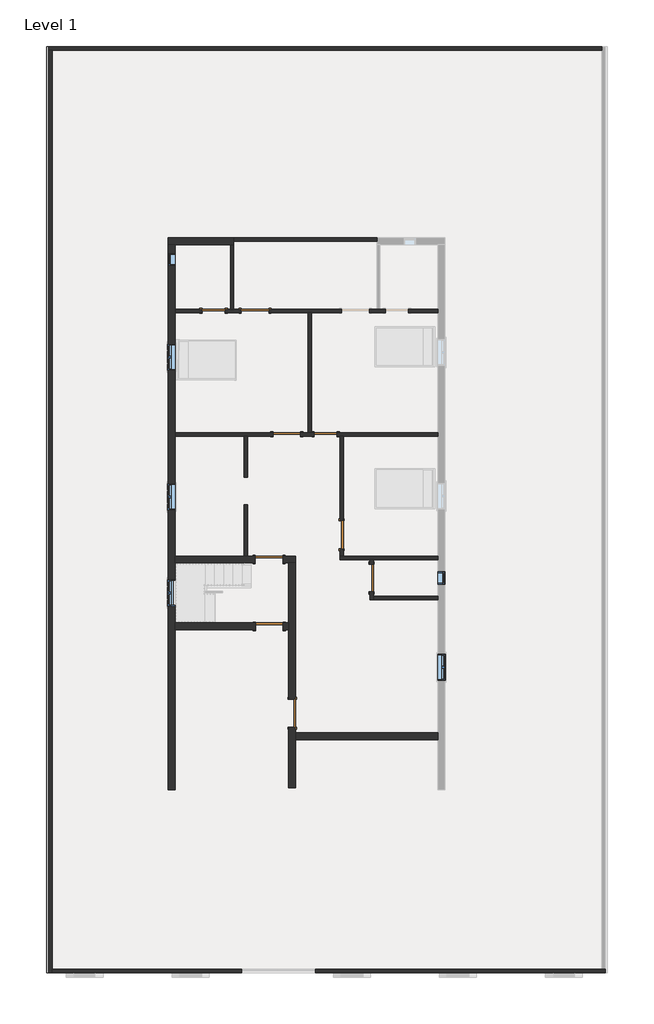
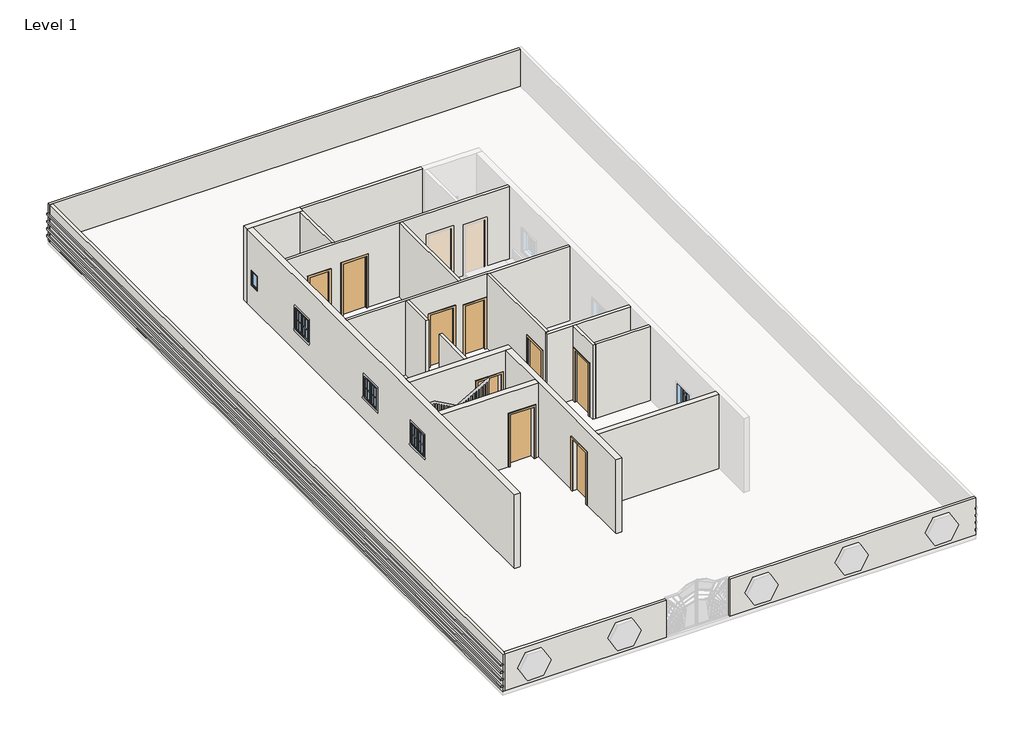
# One storey, part 1 of 3: 21 walls, 9 doors, 6 windows, 4 proxies.
"""IFC4 building model written with IfcOpenShell, lengths in millimetres."""

from ifc_helpers import new_model, si_unit, frame, origin, origin_with_axes, place, context, project, spatial, polyline, outline, extrude, faceted_brep, transform, mapped, element, save
from components import door_d8f5dbb5, door_f2b275c1, door_e5f9f3c4, door_0ca8825f, door_305aa2a5, window_aa618e30, window_339605e1

model = new_model("IFC4")

# Units and contexts
model_context = context("Model", 3, world=origin())
ifc_project = project(units=[si_unit("LENGTHUNIT", "METRE", prefix="MILLI")], contexts=[model_context])

# Site, building, storey
site = spatial("IfcSite", under=ifc_project)
building = spatial("IfcBuilding", under=site)
storey = spatial("IfcBuildingStorey", under=building, Name="Level 1", Elevation=0.0)

# Proxies
placement = place(None, origin())
element("IfcBuildingElementProxy", 1, Name="Reveal", ObjectType="Reveal", at=placement, inside=storey, context=model_context, shape_type="SweptSolid", body=[
    extrude(outline(polyline([(-9754.4734646, -13853.8284905), (-9846.5484646, -13853.8284905), (-9846.5484646, 16740.4715095), (-9754.4734646, 16740.4715095), (-9754.4734646, -13853.8284905)])), frame((0.0, 0.0, 1066.8), z_axis=(0.0, 0.0, 1.0), x_axis=(1.0, 0.0, 0.0)), (0.0, 0.0, 1.0), 67.7333333),
])
element("IfcBuildingElementProxy", 2, Name="Reveal", ObjectType="Reveal", at=placement, inside=storey, context=model_context, shape_type="SweptSolid", body=[
    extrude(outline(polyline([(-9754.4734646, -13853.8284905), (-9846.5484646, -13853.8284905), (-9846.5484646, 16740.4715095), (-9754.4734646, 16740.4715095), (-9754.4734646, -13853.8284905)])), frame((0.0, 0.0, 765.4296979), z_axis=(0.0, 0.0, 1.0), x_axis=(1.0, 0.0, 0.0)), (0.0, 0.0, 1.0), 67.7333333),
])
element("IfcBuildingElementProxy", 3, Name="Reveal", ObjectType="Reveal", at=placement, inside=storey, context=model_context, shape_type="SweptSolid", body=[
    extrude(outline(polyline([(-9754.4734646, -13853.8284905), (-9846.5484646, -13853.8284905), (-9846.5484646, 16740.4715095), (-9754.4734646, 16740.4715095), (-9754.4734646, -13853.8284905)])), frame((0.0, 0.0, 464.0593958), z_axis=(0.0, 0.0, 1.0), x_axis=(1.0, 0.0, 0.0)), (0.0, 0.0, 1.0), 67.7333333),
])
element("IfcBuildingElementProxy", 4, Name="Reveal", ObjectType="Reveal", at=placement, inside=storey, context=model_context, shape_type="SweptSolid", body=[
    extrude(outline(polyline([(-9754.4734646, -13853.8284905), (-9846.5484646, -13853.8284905), (-9846.5484646, 16740.4715095), (-9754.4734646, 16740.4715095), (-9754.4734646, -13853.8284905)])), frame((0.0, 0.0, 174.9956289), z_axis=(0.0, 0.0, 1.0), x_axis=(1.0, 0.0, 0.0)), (0.0, 0.0, 1.0), 67.7333333),
])

# Doors
door_shape = door_d8f5dbb5(model_context)
element("IfcDoor", 5, ObjectType="Single-Flush : 30\" x 80\"", at=placement, inside=storey, context=model_context, shape_type="MappedRepresentation", body=[
    mapped(door_shape, transform((-4322.2915084, 8007.7072267, 0.0), x_axis=(1.0, 0.0, 0.0), y_axis=(0.0, 1.0, 0.0), z_axis=(0.0, 0.0, 1.0))),
])
door_2_shape = door_f2b275c1(model_context)
element("IfcDoor", 6, ObjectType="Single-Flush : 30\" x 80\"", at=placement, inside=storey, context=model_context, shape_type="MappedRepresentation", body=[
    mapped(door_2_shape, transform((-621.124692, 3931.0072267, 0.0), x_axis=(-1.0, 0.0, 0.0), y_axis=(0.0, -1.0, 0.0), z_axis=(0.0, 0.0, 1.0))),
])
door_3_shape = door_e5f9f3c4(model_context)
element("IfcDoor", 7, ObjectType="Single-Flush : 36\" x 84\"", at=placement, inside=storey, context=model_context, shape_type="MappedRepresentation", body=[
    mapped(door_3_shape, transform((-1909.2915084, 3931.0072267, 0.0), x_axis=(1.0, 0.0, 0.0), y_axis=(0.0, 1.0, 0.0), z_axis=(0.0, 0.0, 1.0))),
])
element("IfcDoor", 8, ObjectType="Single-Flush : 36\" x 84\"", at=placement, inside=storey, context=model_context, shape_type="MappedRepresentation", body=[
    mapped(door_3_shape, transform((-94.9578757, 616.3072267, 0.0), x_axis=(0.0, -1.0, 0.0), y_axis=(1.0, 0.0, 0.0), z_axis=(0.0, 0.0, 1.0))),
])
door_4_shape = door_0ca8825f(model_context)
element("IfcDoor", 9, ObjectType="Single-Flush : 36\" x 84\"", at=placement, inside=storey, context=model_context, shape_type="MappedRepresentation", body=[
    mapped(door_4_shape, transform((-2490.3165084, -202.8427733, 0.0), x_axis=(1.0, 0.0, 0.0), y_axis=(0.0, 1.0, 0.0), z_axis=(0.0, 0.0, 1.0))),
])
element("IfcDoor", 10, ObjectType="Single-Flush : 36\" x 84\"", at=placement, inside=storey, context=model_context, shape_type="MappedRepresentation", body=[
    mapped(door_4_shape, transform((-2487.1415084, -2412.6427733, 0.0), x_axis=(1.0, 0.0, 0.0), y_axis=(0.0, 1.0, 0.0), z_axis=(0.0, 0.0, 1.0))),
])
element("IfcDoor", 11, ObjectType="Single-Flush : 36\" x 84\"", at=placement, inside=storey, context=model_context, shape_type="MappedRepresentation", body=[
    mapped(door_4_shape, transform((-1725.1415084, -5282.8427733, 0.0), x_axis=(0.0, -1.0, 0.0), y_axis=(1.0, 0.0, 0.0), z_axis=(0.0, 0.0, 1.0))),
])
door_5_shape = door_305aa2a5(model_context)
element("IfcDoor", 12, ObjectType="Single-Flush : 36\" x 84\"", at=placement, inside=storey, context=model_context, shape_type="MappedRepresentation", body=[
    mapped(door_5_shape, transform((897.4084916, -812.4427733, 0.0), x_axis=(0.0, 1.0, 0.0), y_axis=(-1.0, 0.0, 0.0), z_axis=(0.0, 0.0, 1.0))),
])
element("IfcDoor", 13, ObjectType="Single-Flush : 36\" x 84\"", at=placement, inside=storey, context=model_context, shape_type="MappedRepresentation", body=[
    mapped(door_5_shape, transform((-2950.6915084, 8007.7072267, 0.0), x_axis=(-1.0, 0.0, 0.0), y_axis=(0.0, -1.0, 0.0), z_axis=(0.0, 0.0, 1.0))),
])

# Walls
element("IfcWall", 14, ObjectType="WALL4.5\"", at=placement, inside=storey, context=model_context, shape_type="Brep", body=[
    faceted_brep([(821.2084916, 7950.5572267, 2133.6), (821.2084916, 7950.5572267, 0.0), (1354.6084916, 7950.5572267, 0.0), (1354.6084916, 7950.5572267, 2032.0), (2116.6084916, 7950.5572267, 2032.0), (2116.6084916, 7950.5572267, 0.0), (3088.1584916, 7950.5572267, 0.0), (3088.1584916, 7950.5572267, 3048.0), (-1090.1415084, 7950.5572267, 3048.0), (-1204.4415084, 7950.5572267, 3048.0), (-5598.6415084, 7950.5572267, 3048.0), (-5598.6415084, 7950.5572267, 0.0), (-4703.2915084, 7950.5572267, 0.0), (-4703.2915084, 7950.5572267, 2032.0), (-3941.2915084, 7950.5572267, 2032.0), (-3941.2915084, 7950.5572267, 0.0), (-3407.8915084, 7950.5572267, 0.0), (-3407.8915084, 7950.5572267, 2133.6), (-2493.4915084, 7950.5572267, 2133.6), (-2493.4915084, 7950.5572267, 0.0), (-1204.4415084, 7950.5572267, 0.0), (-1090.1415084, 7950.5572267, 0.0), (-93.1915084, 7950.5572267, 0.0), (-93.1915084, 7950.5572267, 2133.6), (1354.6084916, 8064.8572267, 0.0), (1183.1584916, 8064.8572267, 0.0), (1068.8584916, 8064.8572267, 0.0), (821.2084916, 8064.8572267, 0.0), (821.2084916, 8064.8572267, 2133.6), (-93.1915084, 8064.8572267, 2133.6), (-93.1915084, 8064.8572267, 0.0), (-2493.4915084, 8064.8572267, 0.0), (-2493.4915084, 8064.8572267, 2133.6), (-3407.8915084, 8064.8572267, 2133.6), (-3407.8915084, 8064.8572267, 0.0), (-3655.5415084, 8064.8572267, 0.0), (-3769.8415084, 8064.8572267, 0.0), (-3941.2915084, 8064.8572267, 0.0), (-3941.2915084, 8064.8572267, 2032.0), (-4703.2915084, 8064.8572267, 2032.0), (-4703.2915084, 8064.8572267, 0.0), (-5598.6415084, 8064.8572267, 0.0), (-5598.6415084, 8064.8572267, 3048.0), (-3769.8415084, 8064.8572267, 3048.0), (-3655.5415084, 8064.8572267, 3048.0), (1068.8584916, 8064.8572267, 3048.0), (1183.1584916, 8064.8572267, 3048.0), (3088.1584916, 8064.8572267, 3048.0), (3088.1584916, 8064.8572267, 0.0), (2116.6084916, 8064.8572267, 0.0), (2116.6084916, 8064.8572267, 2032.0), (1354.6084916, 8064.8572267, 2032.0)], [[[0, 1, 2, 3, 4, 5, 6, 7, 8, 9, 10, 11, 12, 13, 14, 15, 16, 17, 18, 19, 20, 21, 22, 23]], [[24, 25, 26, 27, 28, 29, 30, 31, 32, 33, 34, 35, 36, 37, 38, 39, 40, 41, 42, 43, 44, 45, 46, 47, 48, 49, 50, 51]], [[12, 11, 41, 40]], [[49, 48, 6, 5]], [[37, 36, 35, 34, 16, 15]], [[2, 1, 27, 26, 25, 24]], [[22, 21, 20, 19, 31, 30]], [[11, 10, 42, 41]], [[7, 6, 48, 47]], [[38, 37, 15, 14]], [[39, 38, 14, 13]], [[40, 39, 13, 12]], [[3, 2, 24, 51]], [[4, 3, 51, 50]], [[5, 4, 50, 49]], [[17, 16, 34, 33]], [[18, 17, 33, 32]], [[19, 18, 32, 31]], [[28, 27, 1, 0]], [[29, 28, 0, 23]], [[30, 29, 23, 22]], [[10, 9, 8, 7, 47, 46, 45, 44, 43, 42]]]),
])
element("IfcWall", 15, ObjectType="WALL4.5\"", at=placement, inside=storey, context=model_context, shape_type="SweptSolid", body=[
    extrude(outline(polyline([(-3769.8415084, 8064.8572267), (-3769.8415084, 10198.4572267), (-3655.5415084, 10198.4572267), (-3655.5415084, 8064.8572267), (-3769.8415084, 8064.8572267)])), origin_with_axes(), (0.0, 0.0, 1.0), 3048.0),
])
element("IfcWall", 16, ObjectType="WALL4.5\"", at=placement, inside=storey, context=model_context, shape_type="SweptSolid", body=[
    extrude(outline(polyline([(-1204.4415084, 3988.1572267), (-1204.4415084, 7950.5572267), (-1090.1415084, 7950.5572267), (-1090.1415084, 3988.1572267), (-1204.4415084, 3988.1572267)])), origin_with_axes(), (0.0, 0.0, 1.0), 3048.0),
])
element("IfcWall", 17, ObjectType="WALL4.5\"", at=placement, inside=storey, context=model_context, shape_type="Brep", body=[
    faceted_brep([(-1452.0915084, 3873.8572267, 0.0), (-1002.124692, 3873.8572267, 0.0), (-1002.124692, 3873.8572267, 2032.0), (-240.124692, 3873.8572267, 2032.0), (-240.124692, 3873.8572267, 0.0), (-152.1078757, 3873.8572267, 0.0), (-37.8078757, 3873.8572267, 0.0), (3088.1584916, 3873.8572267, 0.0), (3088.1584916, 3873.8572267, 3048.0), (-37.8078757, 3873.8572267, 3048.0), (-152.1078757, 3873.8572267, 3048.0), (-3198.3415084, 3873.8572267, 3048.0), (-3312.6415084, 3873.8572267, 3048.0), (-5598.6415084, 3873.8572267, 3048.0), (-5598.6415084, 3873.8572267, 0.0), (-3312.6415084, 3873.8572267, 0.0), (-3198.3415084, 3873.8572267, 0.0), (-2366.4915084, 3873.8572267, 0.0), (-2366.4915084, 3873.8572267, 2133.6), (-1452.0915084, 3873.8572267, 2133.6), (-1002.124692, 3988.1572267, 2032.0), (-1002.124692, 3988.1572267, 0.0), (-1090.1415084, 3988.1572267, 0.0), (-1204.4415084, 3988.1572267, 0.0), (-1452.0915084, 3988.1572267, 0.0), (-1452.0915084, 3988.1572267, 2133.6), (-2366.4915084, 3988.1572267, 2133.6), (-2366.4915084, 3988.1572267, 0.0), (-5598.6415084, 3988.1572267, 0.0), (-5598.6415084, 3988.1572267, 3048.0), (-1204.4415084, 3988.1572267, 3048.0), (-1090.1415084, 3988.1572267, 3048.0), (3088.1584916, 3988.1572267, 3048.0), (3088.1584916, 3988.1572267, 0.0), (-240.124692, 3988.1572267, 0.0), (-240.124692, 3988.1572267, 2032.0)], [[[0, 1, 2, 3, 4, 5, 6, 7, 8, 9, 10, 11, 12, 13, 14, 15, 16, 17, 18, 19]], [[20, 21, 22, 23, 24, 25, 26, 27, 28, 29, 30, 31, 32, 33, 34, 35]], [[17, 16, 15, 14, 28, 27]], [[34, 33, 7, 6, 5, 4]], [[24, 23, 22, 21, 1, 0]], [[14, 13, 29, 28]], [[8, 7, 33, 32]], [[25, 24, 0, 19]], [[26, 25, 19, 18]], [[27, 26, 18, 17]], [[2, 1, 21, 20]], [[3, 2, 20, 35]], [[4, 3, 35, 34]], [[13, 12, 11, 10, 9, 8, 32, 31, 30, 29]]]),
])
element("IfcWall", 18, ObjectType="WALL4.5\"", at=placement, inside=storey, context=model_context, shape_type="SweptSolid", body=[
    extrude(outline(polyline([(-3312.6415084, 2514.5843832), (-3312.6415084, 3873.8572267), (-3198.3415084, 3873.8572267), (-3198.3415084, 2514.5843832), (-3312.6415084, 2514.5843832)])), origin_with_axes(), (0.0, 0.0, 1.0), 3048.0),
])
element("IfcWall", 19, ObjectType="WALL4.5\"", at=placement, inside=storey, context=model_context, shape_type="SweptSolid", body=[
    extrude(outline(polyline([(-3312.6415084, -88.5427733), (-3312.6415084, 1600.2092553), (-3198.3415084, 1600.2092553), (-3198.3415084, -88.5427733), (-3312.6415084, -88.5427733)])), origin_with_axes(), (0.0, 0.0, 1.0), 3048.0),
])
element("IfcWall", 20, ObjectType="WALL4.5\"", at=placement, inside=storey, context=model_context, shape_type="SweptSolid", body=[
    extrude(outline(polyline([(159.1072267, 2133.6), (159.1072267, 0.0), (-88.5427733, 0.0), (-88.5427733, 3048.0), (3873.8572267, 3048.0), (3873.8572267, 0.0), (1073.5072267, 0.0), (1073.5072267, 2133.6), (159.1072267, 2133.6)])), frame((-152.1078757, 0.0, 0.0), z_axis=(1.0, 0.0, 0.0), x_axis=(0.0, 1.0, 0.0)), (0.0, 0.0, 1.0), 114.3),
])
element("IfcWall", 21, ObjectType="WALL4.5\"", at=placement, inside=storey, context=model_context, shape_type="Brep", body=[
    faceted_brep([(-152.1078757, -202.8427733, 0.0), (840.2584916, -202.8427733, 0.0), (954.5584916, -202.8427733, 0.0), (3088.1584916, -202.8427733, 0.0), (3088.1584916, -202.8427733, 3048.0), (954.5584916, -202.8427733, 3048.0), (840.2584916, -202.8427733, 3048.0), (-152.1078757, -202.8427733, 3048.0), (-152.1078757, -88.5427733, 0.0), (-152.1078757, -88.5427733, 3048.0), (-37.8078757, -88.5427733, 3048.0), (3088.1584916, -88.5427733, 3048.0), (3088.1584916, -88.5427733, 0.0), (-37.8078757, -88.5427733, 0.0)], [[[0, 1, 2, 3, 4, 5, 6, 7]], [[8, 9, 10, 11, 12, 13]], [[3, 2, 1, 0, 8, 13, 12]], [[4, 3, 12, 11]], [[0, 7, 9, 8]], [[7, 6, 5, 4, 11, 10, 9]]]),
])
element("IfcWall", 22, ObjectType="WALL4.5\"", at=placement, inside=storey, context=model_context, shape_type="Brep", body=[
    faceted_brep([(840.2584916, -202.8427733, 0.0), (840.2584916, -355.2427733, 0.0), (840.2584916, -355.2427733, 2133.6), (840.2584916, -1269.6427733, 2133.6), (840.2584916, -1269.6427733, 0.0), (840.2584916, -1536.3427733, 0.0), (840.2584916, -1536.3427733, 3048.0), (840.2584916, -202.8427733, 3048.0), (954.5584916, -355.2427733, 2133.6), (954.5584916, -355.2427733, 0.0), (954.5584916, -202.8427733, 0.0), (954.5584916, -202.8427733, 3048.0), (954.5584916, -1422.0427733, 3048.0), (954.5584916, -1536.3427733, 3048.0), (954.5584916, -1536.3427733, 0.0), (954.5584916, -1422.0427733, 0.0), (954.5584916, -1269.6427733, 0.0), (954.5584916, -1269.6427733, 2133.6)], [[[0, 1, 2, 3, 4, 5, 6, 7]], [[8, 9, 10, 11, 12, 13, 14, 15, 16, 17]], [[10, 9, 1, 0]], [[16, 15, 14, 5, 4]], [[0, 7, 11, 10]], [[6, 5, 14, 13]], [[2, 1, 9, 8]], [[3, 2, 8, 17]], [[4, 3, 17, 16]], [[7, 6, 13, 12, 11]]]),
])
element("IfcWall", 23, ObjectType="WALL4.5\"", at=placement, inside=storey, context=model_context, shape_type="SweptSolid", body=[
    extrude(outline(polyline([(3088.1584916, -1536.3427733), (954.5584916, -1536.3427733), (954.5584916, -1422.0427733), (3088.1584916, -1422.0427733), (3088.1584916, -1536.3427733)])), origin_with_axes(), (0.0, 0.0, 1.0), 3048.0),
])
element("IfcWall", 24, ObjectType="WALL4.5\"", at=placement, inside=storey, context=model_context, shape_type="Brep", body=[
    faceted_brep([(-9779.8734646, 16626.1715095, 0.0), (-9665.5734646, 16626.1715095, 0.0), (8508.1265354, 16626.1715095, 0.0), (8508.1265354, 16626.1715095, 1524.0), (-9665.5734646, 16626.1715095, 1524.0), (-9779.8734646, 16626.1715095, 1524.0), (-9779.8734646, 16626.1715095, 1134.5333333), (-9754.4734646, 16626.1715095, 1134.5333333), (-9754.4734646, 16626.1715095, 1066.8), (-9779.8734646, 16626.1715095, 1066.8), (-9779.8734646, 16626.1715095, 833.1630313), (-9754.4734646, 16626.1715095, 833.1630313), (-9754.4734646, 16626.1715095, 765.4296979), (-9779.8734646, 16626.1715095, 765.4296979), (-9779.8734646, 16626.1715095, 531.7927292), (-9754.4734646, 16626.1715095, 531.7927292), (-9754.4734646, 16626.1715095, 464.0593958), (-9779.8734646, 16626.1715095, 464.0593958), (-9779.8734646, 16626.1715095, 242.7289623), (-9754.4734646, 16626.1715095, 242.7289623), (-9754.4734646, 16626.1715095, 174.9956289), (-9779.8734646, 16626.1715095, 174.9956289), (8508.1265354, 16740.4715095, 0.0), (-9779.8734646, 16740.4715095, 0.0), (-9779.8734646, 16740.4715095, 174.9956289), (-9754.4734646, 16740.4715095, 174.9956289), (-9754.4734646, 16740.4715095, 242.7289623), (-9779.8734646, 16740.4715095, 242.7289623), (-9779.8734646, 16740.4715095, 464.0593958), (-9754.4734646, 16740.4715095, 464.0593958), (-9754.4734646, 16740.4715095, 531.7927292), (-9779.8734646, 16740.4715095, 531.7927292), (-9779.8734646, 16740.4715095, 765.4296979), (-9754.4734646, 16740.4715095, 765.4296979), (-9754.4734646, 16740.4715095, 833.1630313), (-9779.8734646, 16740.4715095, 833.1630313), (-9779.8734646, 16740.4715095, 1066.8), (-9754.4734646, 16740.4715095, 1066.8), (-9754.4734646, 16740.4715095, 1134.5333333), (-9779.8734646, 16740.4715095, 1134.5333333), (-9779.8734646, 16740.4715095, 1524.0), (8508.1265354, 16740.4715095, 1524.0)], [[[0, 1, 2, 3, 4, 5, 6, 7, 8, 9, 10, 11, 12, 13, 14, 15, 16, 17, 18, 19, 20, 21]], [[22, 23, 24, 25, 26, 27, 28, 29, 30, 31, 32, 33, 34, 35, 36, 37, 38, 39, 40, 41]], [[2, 1, 0, 23, 22]], [[5, 4, 3, 41, 40]], [[5, 40, 39, 6]], [[23, 0, 21, 24]], [[9, 36, 35, 10]], [[13, 32, 31, 14]], [[17, 28, 27, 18]], [[3, 2, 22, 41]], [[38, 7, 6, 39]], [[8, 37, 36, 9]], [[7, 38, 37, 8]], [[34, 11, 10, 35]], [[12, 33, 32, 13]], [[11, 34, 33, 12]], [[30, 15, 14, 31]], [[16, 29, 28, 17]], [[15, 30, 29, 16]], [[26, 19, 18, 27]], [[20, 25, 24, 21]], [[19, 26, 25, 20]]]),
])
element("IfcWall", 25, ObjectType="WALL4.5\"", at=placement, inside=storey, context=model_context, shape_type="Brep", body=[
    faceted_brep([(-9665.5734646, -13853.8284905, 0.0), (-9665.5734646, -13739.5284905, 0.0), (-9665.5734646, 16626.1715095, 0.0), (-9665.5734646, 16626.1715095, 1524.0), (-9665.5734646, -13739.5284905, 1524.0), (-9665.5734646, -13853.8284905, 1524.0), (-9779.8734646, 16626.1715095, 0.0), (-9779.8734646, -13853.8284905, 0.0), (-9779.8734646, -13853.8284905, 174.9956289), (-9779.8734646, 16626.1715095, 174.9956289), (-9779.8734646, -13853.8284905, 1524.0), (-9779.8734646, 16626.1715095, 1524.0), (-9779.8734646, 16626.1715095, 1134.5333333), (-9779.8734646, -13853.8284905, 1134.5333333), (-9779.8734646, -13853.8284905, 1066.8), (-9779.8734646, 16626.1715095, 1066.8), (-9779.8734646, 16626.1715095, 833.1630313), (-9779.8734646, -13853.8284905, 833.1630313), (-9779.8734646, -13853.8284905, 765.4296979), (-9779.8734646, 16626.1715095, 765.4296979), (-9779.8734646, 16626.1715095, 531.7927292), (-9779.8734646, -13853.8284905, 531.7927292), (-9779.8734646, -13853.8284905, 464.0593958), (-9779.8734646, 16626.1715095, 464.0593958), (-9779.8734646, 16626.1715095, 242.7289623), (-9779.8734646, -13853.8284905, 242.7289623), (-9754.4734646, -13853.8284905, 1134.5333333), (-9754.4734646, -13853.8284905, 1066.8), (-9754.4734646, -13853.8284905, 833.1630313), (-9754.4734646, -13853.8284905, 765.4296979), (-9754.4734646, -13853.8284905, 531.7927292), (-9754.4734646, -13853.8284905, 464.0593958), (-9754.4734646, -13853.8284905, 242.7289623), (-9754.4734646, -13853.8284905, 174.9956289), (-9754.4734646, 16626.1715095, 174.9956289), (-9754.4734646, 16626.1715095, 242.7289623), (-9754.4734646, 16626.1715095, 464.0593958), (-9754.4734646, 16626.1715095, 531.7927292), (-9754.4734646, 16626.1715095, 765.4296979), (-9754.4734646, 16626.1715095, 833.1630313), (-9754.4734646, 16626.1715095, 1066.8), (-9754.4734646, 16626.1715095, 1134.5333333)], [[[0, 1, 2, 3, 4, 5]], [[6, 7, 8, 9]], [[10, 11, 12, 13]], [[14, 15, 16, 17]], [[18, 19, 20, 21]], [[22, 23, 24, 25]], [[2, 1, 0, 7, 6]], [[5, 4, 3, 11, 10]], [[0, 5, 10, 13, 26, 27, 14, 17, 28, 29, 18, 21, 30, 31, 22, 25, 32, 33, 8, 7]], [[3, 2, 6, 9, 34, 35, 24, 23, 36, 37, 20, 19, 38, 39, 16, 15, 40, 41, 12, 11]], [[41, 26, 13, 12]], [[27, 40, 15, 14]], [[26, 41, 40, 27]], [[39, 28, 17, 16]], [[29, 38, 19, 18]], [[28, 39, 38, 29]], [[37, 30, 21, 20]], [[31, 36, 23, 22]], [[30, 37, 36, 31]], [[35, 32, 25, 24]], [[33, 34, 9, 8]], [[32, 35, 34, 33]]]),
])
element("IfcWall", 26, ObjectType="WALL4.5\"", at=placement, inside=storey, context=model_context, shape_type="Brep", body=[
    faceted_brep([(8622.4265354, -13739.5284905, 0.0), (8508.1265354, -13739.5284905, 0.0), (-947.2665084, -13739.5284905, 0.0), (-947.2665084, -13739.5284905, 1524.0), (8508.1265354, -13739.5284905, 1524.0), (8622.4265354, -13739.5284905, 1524.0), (8622.4265354, -13739.5284905, 1134.5333333), (8597.0265354, -13739.5284905, 1134.5333333), (8597.0265354, -13739.5284905, 1066.8), (8622.4265354, -13739.5284905, 1066.8), (8622.4265354, -13739.5284905, 840.4884563), (8597.0265354, -13739.5284905, 840.4884563), (8597.0265354, -13739.5284905, 772.755123), (8622.4265354, -13739.5284905, 772.755123), (8622.4265354, -13739.5284905, 546.4435793), (8597.0265354, -13739.5284905, 546.4435793), (8597.0265354, -13739.5284905, 478.710246), (8622.4265354, -13739.5284905, 478.710246), (8622.4265354, -13739.5284905, 252.3987023), (8597.0265354, -13739.5284905, 252.3987023), (8597.0265354, -13739.5284905, 184.6653689), (8622.4265354, -13739.5284905, 184.6653689), (-947.2665084, -13853.8284905, 0.0), (8622.4265354, -13853.8284905, 0.0), (8622.4265354, -13853.8284905, 184.6653689), (8597.0265354, -13853.8284905, 184.6653689), (8597.0265354, -13853.8284905, 252.3987023), (8622.4265354, -13853.8284905, 252.3987023), (8622.4265354, -13853.8284905, 478.710246), (8597.0265354, -13853.8284905, 478.710246), (8597.0265354, -13853.8284905, 546.4435793), (8622.4265354, -13853.8284905, 546.4435793), (8622.4265354, -13853.8284905, 772.755123), (8597.0265354, -13853.8284905, 772.755123), (8597.0265354, -13853.8284905, 840.4884563), (8622.4265354, -13853.8284905, 840.4884563), (8622.4265354, -13853.8284905, 1066.8), (8597.0265354, -13853.8284905, 1066.8), (8597.0265354, -13853.8284905, 1134.5333333), (8622.4265354, -13853.8284905, 1134.5333333), (8622.4265354, -13853.8284905, 1524.0), (-947.2665084, -13853.8284905, 1524.0)], [[[0, 1, 2, 3, 4, 5, 6, 7, 8, 9, 10, 11, 12, 13, 14, 15, 16, 17, 18, 19, 20, 21]], [[22, 23, 24, 25, 26, 27, 28, 29, 30, 31, 32, 33, 34, 35, 36, 37, 38, 39, 40, 41]], [[2, 1, 0, 23, 22]], [[3, 2, 22, 41]], [[5, 4, 3, 41, 40]], [[5, 40, 39, 6]], [[23, 0, 21, 24]], [[9, 36, 35, 10]], [[13, 32, 31, 14]], [[17, 28, 27, 18]], [[38, 7, 6, 39]], [[8, 37, 36, 9]], [[7, 38, 37, 8]], [[34, 11, 10, 35]], [[12, 33, 32, 13]], [[11, 34, 33, 12]], [[30, 15, 14, 31]], [[16, 29, 28, 17]], [[15, 30, 29, 16]], [[26, 19, 18, 27]], [[20, 25, 24, 21]], [[19, 26, 25, 20]]]),
])
element("IfcWall", 27, ObjectType="WALL4.5\"", at=placement, inside=storey, context=model_context, shape_type="SweptSolid", body=[
    extrude(outline(polyline([(-9665.5734646, -13739.5284905), (-3404.7165084, -13739.5284905), (-3404.7165084, -13853.8284905), (-9665.5734646, -13853.8284905), (-9665.5734646, -13739.5284905)])), origin_with_axes(), (0.0, 0.0, 1.0), 1524.0),
])
element("IfcWall", 28, ObjectType="WALL4.5\"", at=placement, inside=storey, context=model_context, shape_type="SweptSolid", body=[
    extrude(outline(polyline([(1068.8584916, 10312.7572267), (-3655.5415084, 10312.7572267), (-3655.5415084, 10427.0572267), (1068.8584916, 10427.0572267), (1068.8584916, 10312.7572267)])), origin_with_axes(), (0.0, 0.0, 1.0), 3048.0),
])
element("IfcWall", 29, ObjectType="WALL9\"", at=placement, inside=storey, context=model_context, shape_type="Brep", body=[
    faceted_brep([(-3655.5415084, 10427.0572267, 0.0), (-5827.2415084, 10427.0572267, 0.0), (-5827.2415084, 10427.0572267, 3048.0), (-3655.5415084, 10427.0572267, 3048.0), (-3655.5415084, 10198.4572267, 0.0), (-3655.5415084, 10198.4572267, 3048.0), (-3769.8415084, 10198.4572267, 3048.0), (-5598.6415084, 10198.4572267, 3048.0), (-5827.2415084, 10198.4572267, 3048.0), (-5827.2415084, 10198.4572267, 0.0), (-5598.6415084, 10198.4572267, 0.0), (-3769.8415084, 10198.4572267, 0.0), (-3655.5415084, 10312.7572267, 0.0), (-3655.5415084, 10312.7572267, 3048.0)], [[[0, 1, 2, 3]], [[4, 5, 6, 7, 8, 9, 10, 11]], [[1, 0, 12, 4, 11, 10, 9]], [[2, 1, 9, 8]], [[0, 3, 13, 5, 4, 12]], [[3, 2, 8, 7, 6, 5, 13]]]),
])
element("IfcWall", 30, ObjectType="WALL9\"", at=placement, inside=storey, context=model_context, shape_type="Brep", body=[
    faceted_brep([(-5827.2415084, 10198.4572267, 0.0), (-5827.2415084, -7803.7927733, 0.0), (-5827.2415084, -7803.7927733, 3048.0), (-5827.2415084, 10198.4572267, 3048.0), (-5827.2415084, 9906.3572267, 1524.0), (-5827.2415084, 9499.9572267, 1524.0), (-5827.2415084, 9499.9572267, 914.4), (-5827.2415084, 9906.3572267, 914.4), (-5827.2415084, 6915.5072267, 1828.8), (-5827.2415084, 6051.9072267, 1828.8), (-5827.2415084, 6051.9072267, 914.4), (-5827.2415084, 6915.5072267, 914.4), (-5827.2415084, 2295.8822267, 1828.8), (-5827.2415084, 1432.2822267, 1828.8), (-5827.2415084, 1432.2822267, 914.4), (-5827.2415084, 2295.8822267, 914.4), (-5827.2415084, -875.9427733, 1828.8), (-5827.2415084, -1739.5427733, 1828.8), (-5827.2415084, -1739.5427733, 914.4), (-5827.2415084, -875.9427733, 914.4), (-5598.6415084, 10198.4572267, 0.0), (-5598.6415084, 10198.4572267, 3048.0), (-5598.6415084, 8064.8572267, 3048.0), (-5598.6415084, 7950.5572267, 3048.0), (-5598.6415084, 3988.1572267, 3048.0), (-5598.6415084, 3873.8572267, 3048.0), (-5598.6415084, -88.5427733, 3048.0), (-5598.6415084, -317.1427733, 3048.0), (-5598.6415084, -2298.3427733, 3048.0), (-5598.6415084, -2526.9427733, 3048.0), (-5598.6415084, -7803.7927733, 3048.0), (-5598.6415084, -7803.7927733, 0.0), (-5598.6415084, -2526.9427733, 0.0), (-5598.6415084, -2298.3427733, 0.0), (-5598.6415084, -317.1427733, 0.0), (-5598.6415084, -88.5427733, 0.0), (-5598.6415084, 3873.8572267, 0.0), (-5598.6415084, 3988.1572267, 0.0), (-5598.6415084, 7950.5572267, 0.0), (-5598.6415084, 8064.8572267, 0.0), (-5598.6415084, 9906.3572267, 1524.0), (-5598.6415084, 9906.3572267, 914.4), (-5598.6415084, 9499.9572267, 914.4), (-5598.6415084, 9499.9572267, 1524.0), (-5598.6415084, 6915.5072267, 1828.8), (-5598.6415084, 6915.5072267, 914.4), (-5598.6415084, 6051.9072267, 914.4), (-5598.6415084, 6051.9072267, 1828.8), (-5598.6415084, 2295.8822267, 1828.8), (-5598.6415084, 2295.8822267, 914.4), (-5598.6415084, 1432.2822267, 914.4), (-5598.6415084, 1432.2822267, 1828.8), (-5598.6415084, -875.9427733, 1828.8), (-5598.6415084, -875.9427733, 914.4), (-5598.6415084, -1739.5427733, 914.4), (-5598.6415084, -1739.5427733, 1828.8)], [[[0, 1, 2, 3], [4, 5, 6, 7], [8, 9, 10, 11], [12, 13, 14, 15], [16, 17, 18, 19]], [[20, 21, 22, 23, 24, 25, 26, 27, 28, 29, 30, 31, 32, 33, 34, 35, 36, 37, 38, 39], [40, 41, 42, 43], [44, 45, 46, 47], [48, 49, 50, 51], [52, 53, 54, 55]], [[1, 0, 20, 39, 38, 37, 36, 35, 34, 33, 32, 31]], [[2, 1, 31, 30]], [[0, 3, 21, 20]], [[41, 40, 4, 7]], [[42, 41, 7, 6]], [[43, 42, 6, 5]], [[40, 43, 5, 4]], [[45, 44, 8, 11]], [[46, 45, 11, 10]], [[47, 46, 10, 9]], [[44, 47, 9, 8]], [[49, 48, 12, 15]], [[50, 49, 15, 14]], [[51, 50, 14, 13]], [[48, 51, 13, 12]], [[53, 52, 16, 19]], [[54, 53, 19, 18]], [[55, 54, 18, 17]], [[52, 55, 17, 16]], [[3, 2, 30, 29, 28, 27, 26, 25, 24, 23, 22, 21]]]),
])
element("IfcWall", 31, ObjectType="WALL9\"", at=placement, inside=storey, context=model_context, shape_type="Brep", body=[
    faceted_brep([(-2033.1165084, -317.1427733, 2133.6), (-2033.1165084, -317.1427733, 0.0), (-1839.4415084, -317.1427733, 0.0), (-1610.8415084, -317.1427733, 0.0), (-1610.8415084, -317.1427733, 3048.0), (-1839.4415084, -317.1427733, 3048.0), (-5598.6415084, -317.1427733, 3048.0), (-5598.6415084, -317.1427733, 0.0), (-2947.5165084, -317.1427733, 0.0), (-2947.5165084, -317.1427733, 2133.6), (-1610.8415084, -88.5427733, 0.0), (-2033.1165084, -88.5427733, 0.0), (-2033.1165084, -88.5427733, 2133.6), (-2947.5165084, -88.5427733, 2133.6), (-2947.5165084, -88.5427733, 0.0), (-3198.3415084, -88.5427733, 0.0), (-3312.6415084, -88.5427733, 0.0), (-5598.6415084, -88.5427733, 0.0), (-5598.6415084, -88.5427733, 3048.0), (-3312.6415084, -88.5427733, 3048.0), (-3198.3415084, -88.5427733, 3048.0), (-1610.8415084, -88.5427733, 3048.0)], [[[0, 1, 2, 3, 4, 5, 6, 7, 8, 9]], [[10, 11, 12, 13, 14, 15, 16, 17, 18, 19, 20, 21]], [[8, 7, 17, 16, 15, 14]], [[3, 2, 1, 11, 10]], [[7, 6, 18, 17]], [[4, 3, 10, 21]], [[12, 11, 1, 0]], [[13, 12, 0, 9]], [[14, 13, 9, 8]], [[6, 5, 4, 21, 20, 19, 18]]]),
])
element("IfcWall", 32, ObjectType="WALL9\"", at=placement, inside=storey, context=model_context, shape_type="Brep", body=[
    faceted_brep([(-1839.4415084, -5740.0427733, 2133.6), (-1839.4415084, -5740.0427733, 0.0), (-1839.4415084, -7733.9427733, 0.0), (-1839.4415084, -7733.9427733, 3048.0), (-1839.4415084, -2526.9427733, 3048.0), (-1839.4415084, -2298.3427733, 3048.0), (-1839.4415084, -317.1427733, 3048.0), (-1839.4415084, -317.1427733, 0.0), (-1839.4415084, -2298.3427733, 0.0), (-1839.4415084, -2526.9427733, 0.0), (-1839.4415084, -4825.6427733, 0.0), (-1839.4415084, -4825.6427733, 2133.6), (-1610.8415084, -7733.9427733, 0.0), (-1610.8415084, -6159.1427733, 0.0), (-1610.8415084, -5930.5427733, 0.0), (-1610.8415084, -5740.0427733, 0.0), (-1610.8415084, -5740.0427733, 2133.6), (-1610.8415084, -4825.6427733, 2133.6), (-1610.8415084, -4825.6427733, 0.0), (-1610.8415084, -317.1427733, 0.0), (-1610.8415084, -317.1427733, 3048.0), (-1610.8415084, -5930.5427733, 3048.0), (-1610.8415084, -6159.1427733, 3048.0), (-1610.8415084, -7733.9427733, 3048.0)], [[[0, 1, 2, 3, 4, 5, 6, 7, 8, 9, 10, 11]], [[12, 13, 14, 15, 16, 17, 18, 19, 20, 21, 22, 23]], [[2, 1, 15, 14, 13, 12]], [[10, 9, 8, 7, 19, 18]], [[3, 2, 12, 23]], [[7, 6, 20, 19]], [[16, 15, 1, 0]], [[17, 16, 0, 11]], [[18, 17, 11, 10]], [[6, 5, 4, 3, 23, 22, 21, 20]]]),
])
element("IfcWall", 33, ObjectType="WALL9\"", at=placement, inside=storey, context=model_context, shape_type="SweptSolid", body=[
    extrude(outline(polyline([(3088.1584916, -6159.1427733), (-1610.8415084, -6159.1427733), (-1610.8415084, -5930.5427733), (3088.1584916, -5930.5427733), (3088.1584916, -6159.1427733)])), origin_with_axes(), (0.0, 0.0, 1.0), 3048.0),
])
element("IfcWall", 34, ObjectType="WALL9\"", at=placement, inside=storey, context=model_context, shape_type="SweptSolid", body=[
    extrude(outline(polyline([(2133.6, -2029.9415084), (0.0, -2029.9415084), (0.0, -1839.4415084), (3048.0, -1839.4415084), (3048.0, -5598.6415084), (0.0, -5598.6415084), (0.0, -2944.3415084), (2133.6, -2944.3415084), (2133.6, -2029.9415084)])), frame((0.0, -2526.9427733, 0.0), z_axis=(0.0, 1.0, 0.0), x_axis=(0.0, 0.0, 1.0)), (0.0, 0.0, 1.0), 228.6),
])

# Windows
window_shape = window_aa618e30(model_context)
element("IfcWindow", 35, ObjectType="Fixed : 16\" x 24\"", at=placement, inside=storey, context=model_context, shape_type="MappedRepresentation", body=[
    mapped(window_shape, transform((-5712.9415084, 9741.2572267, 0.0), x_axis=(0.0, 1.0, 0.0), y_axis=(-1.0, 0.0, 0.0), z_axis=(0.0, 0.0, 1.0))),
])
element("IfcWindow", 36, ObjectType="Fixed : 16\" x 24\"", at=placement, inside=storey, context=model_context, shape_type="MappedRepresentation", body=[
    mapped(window_shape, transform((3202.4584916, -850.5427733, 0.0), x_axis=(0.0, -1.0, 0.0), y_axis=(1.0, 0.0, 0.0), z_axis=(0.0, 0.0, 1.0))),
])
window_2_shape = window_339605e1(model_context)
element("IfcWindow", 37, ObjectType="Window-Casement-Double : 34\" x 36\"", at=placement, inside=storey, context=model_context, shape_type="MappedRepresentation", body=[
    mapped(window_2_shape, transform((-5712.9415084, 6483.7072267, 0.0), x_axis=(0.0, 1.0, 0.0), y_axis=(-1.0, 0.0, 0.0), z_axis=(0.0, 0.0, 1.0))),
])
element("IfcWindow", 38, ObjectType="Window-Casement-Double : 34\" x 36\"", at=placement, inside=storey, context=model_context, shape_type="MappedRepresentation", body=[
    mapped(window_2_shape, transform((-5712.9415084, 1864.0822267, 0.0), x_axis=(0.0, 1.0, 0.0), y_axis=(-1.0, 0.0, 0.0), z_axis=(0.0, 0.0, 1.0))),
])
element("IfcWindow", 39, ObjectType="Window-Casement-Double : 34\" x 36\"", at=placement, inside=storey, context=model_context, shape_type="MappedRepresentation", body=[
    mapped(window_2_shape, transform((3202.4584916, -3762.0177733, 0.0), x_axis=(0.0, -1.0, 0.0), y_axis=(1.0, 0.0, 0.0), z_axis=(0.0, 0.0, 1.0))),
])
element("IfcWindow", 40, ObjectType="Window-Casement-Double : 34\" x 36\"", at=placement, inside=storey, context=model_context, shape_type="MappedRepresentation", body=[
    mapped(window_2_shape, transform((-5712.9415084, -1307.7427733, 0.0), x_axis=(0.0, 1.0, 0.0), y_axis=(-1.0, 0.0, 0.0), z_axis=(0.0, 0.0, 1.0))),
])

save(model, "model.ifc")

# Revit data of these elements
# Type "Single-Flush : 30\" x 80\""
#   Type Mark = "5"
#   Construction Type Id = "MDOOR"
#   Assembly Code = "C1020"
#   Analytic Construction = "Metal"
#   Thickness = 0' - 2"
#   Heat Transfer Coefficient (U) = 0.651978 BTU/(h·ft²·°F)
#   Height = 6' - 8"
#   Trim Projection Ext = 0' - 1"
#   Trim Projection Int = 0' - 1"
#   Trim Width = 0' - 3"
#   Width = 2' - 6"
#   Define Thermal Properties by = 1
#   Define Thermal Properties by = 1
#   Door Material = Door - Panel
#   Frame Material = Door - Frame
#   Visual Light Transmittance = 0
#   Solar Heat Gain Coefficient = 0
#   Function = (empty or 0)
#   Wall Closure = (empty or 0)
# Type "Single-Flush : 36\" x 84\""
#   Type Mark = "1"
#   Construction Type Id = "MDOOR"
#   Assembly Code = "C1020"
#   Analytic Construction = "Metal"
#   Thickness = 0' - 2"
#   Heat Transfer Coefficient (U) = 0.651978 BTU/(h·ft²·°F)
#   Height = 7' - 0"
#   Trim Projection Ext = 0' - 1"
#   Trim Projection Int = 0' - 1"
#   Trim Width = 0' - 3"
#   Width = 3' - 0"
#   Define Thermal Properties by = 1
#   Define Thermal Properties by = 1
#   Door Material = Door - Panel
#   Frame Material = Door - Frame
#   Visual Light Transmittance = 0
#   Solar Heat Gain Coefficient = 0
#   Function = (empty or 0)
#   Wall Closure = (empty or 0)
# Type "WALL4.5\""
#   Assembly Code = "B2010"
#   Layers, outside or top first: 0' - 4 1/2" no material (function 1)
# Type "WALL9\""
#   Assembly Code = "B2010"
#   Layers, outside or top first: 0' - 9" no material (function 1)
# Type "Fixed : 16\" x 24\""
#   Type Mark = "4"
#   Construction Type Id = "GSP4R"
#   Assembly Code = "B2020100"
#   Analytic Construction = "1/8 in Pilkington single glazing"
#   Visual Light Transmittance = 0.9
#   Solar Heat Gain Coefficient = 0.78
#   Heat Transfer Coefficient (U) = 0.6496 BTU/(h·ft²·°F)
#   Height = 2' - 0"
#   Default Sill Height = 3' - 0"
#   Width = 1' - 4"
#   Window Inset = 0' - 0 3/4"
#   Define Thermal Properties by = 1
#   Define Thermal Properties by = 1
#   Glass Pane Material = Glass
#   Sash Material = Sash
#   Wall Closure = (empty or 0)
# Type "Window-Casement-Double : 34\" x 36\""
#   Type Mark = "14"
#   Fire Rating = "0.5h"
#   Assembly Code = "B2020100"
#   Analytic Construction = "Double glazing - domestic"
#   Frame Extension [instance default] = 0' - 0 1/4"
#   Window Inset [instance default] = 0' - 0"
#   Wall Thickness [instance default] = 0' - 6"
#   Interior Wall Closure [instance default] = 0' - 2 1/4"
#   Half Width = 1' - 5"
#   Visual Light Transmittance = 0.81
#   Thermal Resistance (R) = 1.8146 (h·ft²·°F)/BTU
#   Solar Heat Gain Coefficient = 0.76
#   Rough Width = 2' - 10 1/2"
#   Rough Height = 3' - 0 1/2"
#   Height = 3' - 0"
#   Heat Transfer Coefficient (U) = 0.5511 BTU/(h·ft²·°F)
#   Exterior Wall Closure [instance default] = 0' - 1 1/4"
#   Extension Jamb [instance default] = 0' - 2 1/4"
#   Default Sill Height = 3' - 0"
#   Width = 2' - 10"
#   Define Thermal Properties by = 0
#   Muntin Visibility = yes
#   Interior Trim Visibility [instance default] = yes
#   Exterior Trim Visibility [instance default] = yes
#   Extension Jamb Visibility [instance default] = yes
#   Interior Trim Material = Wood - Stained
#   Muntin Pattern = Muntin Pattern_2x2 : Muntin Pattern_2x2
#   Interior Trim = Trim-Window-Interior-Flat : Picture Frame
#   Interior Frame Material = Wood - Stained
#   Glass Panel Material = Glass
#   Exterior Trim Material = Clad - White
#   Exterior Trim = Trim-Window-Exterior-Flat : with Sill
#   Exterior Frame Material = Clad - White
#   Wall Closure = (empty or 0)
# Elements 5, 6 (IfcDoor, "Single-Flush : 30\" x 80\"")
#   Phase Created = New Construction
#   Materials on its faces: "Door - Frame", "Door - Panel"
# Elements 7, 8, 9, 10, 11, 12, 13 (IfcDoor, "Single-Flush : 36\" x 84\"")
#   Phase Created = New Construction
#   Materials on its faces: "Door - Frame", "Door - Panel"
# Elements 14, 28 (IfcWall, "WALL4.5\"")
#   Top Offset = 0' - 0"
#   Base Offset = 0' - 0"
#   Unconnected Height = 10' - 0"
#   wall height = 10' - 0"
#   Phase Created = New Construction
#   Base Constraint = Level 1
#   Materials on its faces: "Default Wall", "Wood Planks"
# Elements 15, 16, 17, 18, 19, 20, 21, 22, 23 (IfcWall, "WALL4.5\"")
#   Top Offset = 0' - 0"
#   Base Offset = 0' - 0"
#   Unconnected Height = 10' - 0"
#   wall height = 10' - 0"
#   Phase Created = New Construction
#   Base Constraint = Level 1
#   Materials on its faces: "Default Wall"
# Elements 24, 25, 26, 27 (IfcWall, "WALL4.5\"")
#   Top Offset = 0' - 0"
#   Base Offset = 0' - 0"
#   Unconnected Height = 5' - 0"
#   wall height = 5' - 0"
#   Phase Created = New Construction
#   Base Constraint = Level 1
#   Materials on its faces: "Default Wall", "Door - Frame"
# Elements 29, 30, 31, 32, 33, 34 (IfcWall, "WALL9\"")
#   Top Offset = 0' - 0"
#   Base Offset = 0' - 0"
#   Unconnected Height = 10' - 0"
#   wall height = 10' - 0"
#   Phase Created = New Construction
#   Base Constraint = Level 1
#   Materials on its faces: "Default Wall", "Wood Planks"
# Element 35 (IfcWindow, "Fixed : 16\" x 24\"")
#   Mark = "1"
#   Phase Created = New Construction
#   Materials on its faces: "Sash", "Glass"
# Element 36 (IfcWindow, "Fixed : 16\" x 24\"")
#   Mark = "3"
#   Phase Created = New Construction
#   Materials on its faces: "Sash", "Glass"
# Element 37 (IfcWindow, "Window-Casement-Double : 34\" x 36\"")
#   Mark = "6"
#   Window Inset = 0' - 0"
#   Interior Wall Closure = 0' - 2 1/4"
#   Frame Extension = 0' - 0 1/4"
#   Exterior Wall Closure = 0' - 1 1/4"
#   Interior Trim Visibility = yes
#   Exterior Trim Visibility = yes
#   Phase Created = New Construction
#   Materials on its faces: "Wood - Stained", "Glass", "Clad - White"
# Element 38 (IfcWindow, "Window-Casement-Double : 34\" x 36\"")
#   Mark = "7"
#   Window Inset = 0' - 0"
#   Interior Wall Closure = 0' - 2 1/4"
#   Frame Extension = 0' - 0 1/4"
#   Exterior Wall Closure = 0' - 1 1/4"
#   Interior Trim Visibility = yes
#   Exterior Trim Visibility = yes
#   Phase Created = New Construction
#   Materials on its faces: "Wood - Stained", "Glass", "Clad - White"
# Element 39 (IfcWindow, "Window-Casement-Double : 34\" x 36\"")
#   Mark = "8"
#   Window Inset = 0' - 0"
#   Interior Wall Closure = 0' - 2 1/4"
#   Frame Extension = 0' - 0 1/4"
#   Exterior Wall Closure = 0' - 1 1/4"
#   Interior Trim Visibility = yes
#   Exterior Trim Visibility = yes
#   Phase Created = New Construction
#   Materials on its faces: "Wood - Stained", "Glass", "Clad - White"
# Element 40 (IfcWindow, "Window-Casement-Double : 34\" x 36\"")
#   Mark = "9"
#   Window Inset = 0' - 0"
#   Interior Wall Closure = 0' - 2 1/4"
#   Frame Extension = 0' - 0 1/4"
#   Exterior Wall Closure = 0' - 1 1/4"
#   Interior Trim Visibility = yes
#   Exterior Trim Visibility = yes
#   Phase Created = New Construction
#   Materials on its faces: "Wood - Stained", "Glass", "Clad - White"
# Materials
#   "Door - Panel": class "Wood", colour RGB 210 159 95, transparency 0, Cost = 0
#   "Door - Frame": colour RGB 118 70 51, transparency 0, Cost = 0
#   "Glass": class "Glass", colour RGB 0 128 192, transparency 0.75, Description = "Soda Lime Glass", Cost = 0
#   "Sash": class "Wood", colour RGB 224 178 126, transparency 0, Cost = 0
#   "Wood - Stained": class "Wood", colour RGB 224 178 126, transparency 0, Cost = 0
#   "Clad - White": class "Wood", colour RGB 242 242 238, transparency 0, Cost = 0
#   "Default Wall": colour RGB 128 128 128, transparency 0, Cost = 0
#   "Wood Planks": class "Wood", colour RGB 193 160 115, transparency 0, Description = "Physical material.", Cost = 0
